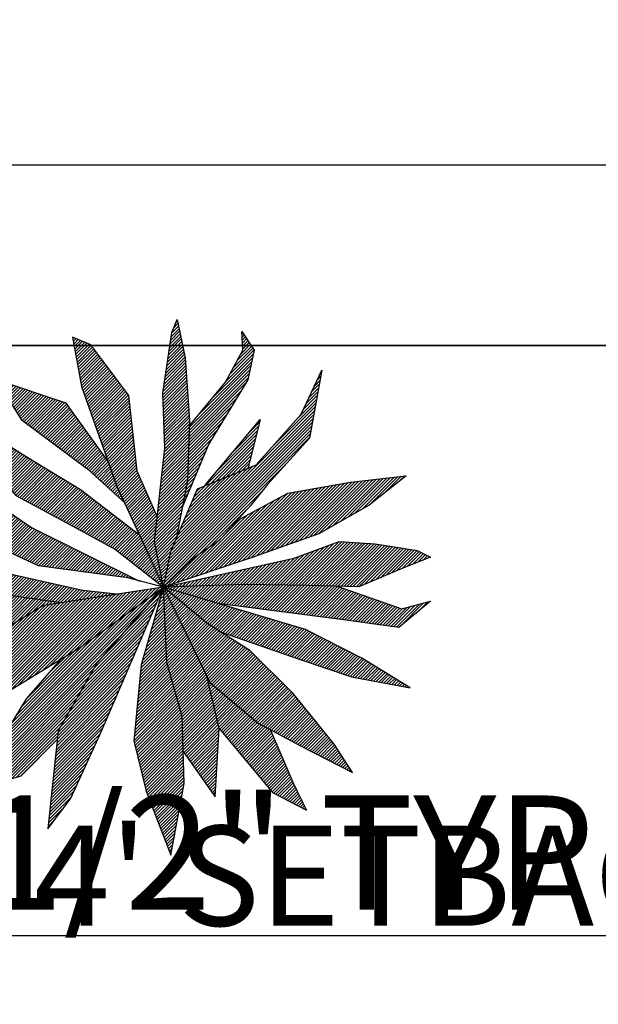
# Model space of a CAD drawing. Units: inches. Extents: x 1986 to 21484, y -1816 to 2016.
# Tile 49 of 85: x 3604 to 3645, y 1855 to 1924. Entities that reach past the tile are written whole.
import ezdxf

# ---------------------------------------------------------------- set-up
doc = ezdxf.new("R2010")
doc.units = ezdxf.units.IN
for name, color, linetype, lineweight in [('A-ANNO-DIMS', 2, 'Continuous', 18), ('A-ANNO-TEXT', 7, 'Continuous', 18), ('C-PROP', 7, 'Continuous', 35), ('L-PLNT', 84, 'Continuous', 13), ('vfolhas', 114, 'Continuous', 5)]:
    doc.layers.add(name, color=color, linetype=linetype, lineweight=lineweight)
for name, color, linetype in [('vfolha', 72, 'Continuous'), ('vfolha2', 110, 'Continuous'), ('vfolhas2', 102, 'Continuous')]:
    doc.layers.add(name, color=color, linetype=linetype)
doc.styles.get("Standard").update_dxf_attribs({"font": 'arial.ttf'})
doc.dimstyles.new('ISO-25', dxfattribs={"dimtxt": 8, "dimasz": 2.5, "dimexe": 1.25, "dimexo": 0.625, "dimtad": 1, "dimdec": 1, "dimlunit": 3, "dimtxsty": 'Standard', "dimcen": 2.5, "dimadec": 0, "dimazin": 0, "dimtfac": 1, "dimtdec": 1, "dimtmove": 0, "dimatfit": 3, "dimfxl": 1, "dimarcsym": 0})
pattern_1 = [(45, (-2446.5133113, 50.986076), (-0.004419417382, 0.004419417382), [])]

# ---------------------------------------------------------------- blocks, each defined once
blk = doc.blocks.new('*D33')
at = {"layer": 'A-ANNO-DIMS', "color": 0, "lineweight": -2, "transparency": 16777216}
for p, q in [((3538.907, 1901.377), (3538.907, 1914.655)), ((3898.907, 1901.377), (3898.907, 1914.655)), ((3541.407, 1913.405), (3896.407, 1913.405))]:
    blk.add_line(p, q, dxfattribs=at)
at = {"layer": 'A-ANNO-DIMS', "color": 0, "transparency": 16777216}
for points in [[(3541.407, 1913.821), (3541.407, 1912.988), (3538.907, 1913.405)], [(3896.407, 1913.821), (3896.407, 1912.988), (3898.907, 1913.405)]]:
    blk.add_solid(points, dxfattribs=at)
at = {"layer": 'Defpoints', "color": 0, "transparency": 16777216}
for p in [(3898.907, 1913.405), (3538.907, 1900.752), (3898.907, 1900.752)]:
    blk.add_point(p, dxfattribs=at)
at = {"layer": 'A-ANNO-DIMS', "color": 0, "transparency": 16777216, "insert": (3718.907, 1918.117), "char_height": 8, "attachment_point": 5}
blk.add_mtext("30'", dxfattribs=at)
blk = doc.blocks.new('arbusto_PB_verde_grande')
at = {"layer": 'vfolha2'}
h = blk.add_hatch(dxfattribs=at)
h.set_pattern_fill('ANSI31', color=256, scale=0.05, style=0)
h.set_pattern_definition(pattern_1)
h.paths.add_polyline_path([(0.0294, 0.3565), (0.0003, 0.0905), (0.0263, -0.0393), (0.047, 0.0623), (0.0619, 0.0973), (0.0937, 0.2657), (0.0996, 0.4347), (0.0879, 0.6131), (0.0645, 0.7227), (0.0499, 0.6851), (0.0236, 0.5129)])
h.paths.add_polyline_path([(0.3011, 0.4379), (0.1423, 0.2487), (0.2669, 0.3002)])
h.paths.add_polyline_path([(0.38, 0.2282), (0.237, 0.1519), (0.1843, 0.0936), (0.1112, 0.0436), (0.0263, -0.0393), (0.2806, 0.0467), (0.3683, 0.078), (0.4676, 0.1124), (0.6107, 0.1938), (0.7159, 0.2782), (0.5581, 0.2595)])
h.paths.add_polyline_path([(0.561, -0.2944), (0.7275, -0.3257), (0.5902, -0.2412), (0.4296, -0.1598), (0.0263, -0.0393), (0.1492, -0.1411), (0.1884, -0.166), (0.415, -0.2444)])
h.paths.add_polyline_path([(-0.2743, -0.4478), (-0.3035, -0.7263), (-0.2392, -0.6417), (-0.1546, -0.4572), (0.0263, -0.0393), (-0.1633, -0.2538)])
h.paths.add_polyline_path([(-0.5196, -0.2474), (-0.6774, -0.3257), (-0.5956, -0.3507), (-0.4057, -0.3288), (-0.2101, -0.21), (0.0263, -0.0393), (-0.1487, -0.0659), (-0.3152, -0.091), (-0.4145, -0.1505)])
h.paths.add_polyline_path([(-0.5255, 0.2501), (-0.7095, 0.247), (-0.5196, 0.1093), (-0.3298, 0.0217), (-0.0757, -0.0128), (-0.0423, -0.0215), (-0.3502, 0.1312)])
h = blk.add_hatch(dxfattribs=at)
h.set_pattern_fill('ANSI31', color=256, scale=0.05, style=0)
h.set_pattern_definition(pattern_1)
h.paths.add_polyline_path([(-0.1896, 0.297), (-0.0855, 0.2019), (-0.1078, 0.2501), (-0.132, 0.3187), (-0.251, 0.4848), (-0.4495, 0.5505), (-0.3795, 0.4379)])
h.paths.add_polyline_path([(0.0791, -0.4071), (0.0821, -0.5063), (0.1726, -0.6355), (0.1843, -0.4415), (0.149, -0.2918), (0.0263, -0.0393), (0.0353, -0.2538)])
at = {"layer": 'vfolhas'}
h = blk.add_hatch(dxfattribs=at)
h.set_pattern_fill('ANSI31', color=256, scale=0.05, style=0)
h.set_pattern_definition(pattern_1)
h.paths.add_polyline_path([(-0.0728, 0.5067), (-0.1808, 0.6506), (-0.2334, 0.6725), (-0.2071, 0.5318), (-0.1078, 0.2501), (0.0263, -0.0393), (0.0003, 0.0905), (0.0082, 0.1624), (-0.0494, 0.2908)])
h.paths.add_polyline_path([(0.099, 0.4193), (0.0937, 0.2657), (0.0791, 0.1881), (0.1551, 0.369), (0.2661, 0.5505), (0.2836, 0.635), (0.2485, 0.6882), (0.2514, 0.635), (0.2018, 0.5443)])
h.paths.add_polyline_path([(0.1229, 0.2407), (0.047, 0.0623), (0.0263, -0.0393), (0.1112, 0.0436), (0.1843, 0.0936), (0.2748, 0.1938), (0.3215, 0.2532), (0.4413, 0.3847), (0.4763, 0.5787), (0.4179, 0.4535), (0.2894, 0.3095)])
h.paths.add_polyline_path([(0.5815, -0.0378), (0.7071, 0.0154), (0.7859, 0.0467), (0.748, 0.0655), (0.6282, 0.0842), (0.526, 0.0905), (0.3974, 0.0436), (0.0263, -0.0393), (0.2573, -0.0315), (0.4383, -0.0347)])
h.paths.add_polyline_path([(0.5202, -0.0365), (0.4383, -0.0347), (0.2573, -0.0315), (0.0263, -0.0393), (0.1796, -0.0852), (0.5377, -0.1317), (0.6954, -0.1536), (0.7859, -0.0785), (0.7041, -0.1004)])
h.paths.add_polyline_path([(0.2719, -0.2193), (0.1492, -0.1411), (0.0263, -0.0393), (0.1579, -0.3101), (0.2952, -0.4258), (0.4179, -0.4916), (0.564, -0.5667), (0.5114, -0.4853), (0.3946, -0.3414)])
h.paths.add_polyline_path([(-0.0582, -0.4759), (-0.0231, -0.6198), (0.047, -0.8013), (0.0849, -0.5979), (0.0791, -0.4071), (0.0353, -0.2538), (0.0263, -0.0393), (-0.0377, -0.26)])
h.paths.add_polyline_path([(-0.2422, 0.1405), (-0.1107, 0.0686), (0.0263, -0.0393), (-0.0423, 0.1087), (-0.2101, 0.2376), (-0.3649, 0.3314), (-0.4787, 0.4034), (-0.543, 0.4629), (-0.4904, 0.3314), (-0.3941, 0.2219)])
h = blk.add_hatch(dxfattribs=at)
h.set_pattern_fill('ANSI31', color=256, scale=0.05, style=0)
h.set_pattern_definition(pattern_1)
h.paths.add_polyline_path([(-0.5722, 0.0623), (-0.7153, 0.103), (-0.6774, 0.0811), (-0.6277, 0.0154), (-0.5635, -0.041), (-0.2646, -0.0834), (-0.1487, -0.0659), (-0.1015, -0.0588), (-0.2042, -0.0472), (-0.4028, -0.0034)])
h.paths.add_polyline_path([(-0.5635, -0.041), (-0.5828, -0.024), (-0.7299, -0.0973), (-0.4334, -0.1679), (-0.4145, -0.1505), (-0.3152, -0.091), (-0.2646, -0.0834)])
h.paths.add_polyline_path([(-0.2769, -0.4727), (-0.2743, -0.4478), (-0.1633, -0.2538), (0.0263, -0.0393), (-0.2101, -0.21), (-0.2672, -0.2447), (-0.3649, -0.357), (-0.4291, -0.4634), (-0.4759, -0.6043), (-0.3795, -0.576)])
h = blk.add_hatch(dxfattribs=at)
h.set_pattern_fill('ANSI31', color=256, scale=0.05, style=0)
h.set_pattern_definition(pattern_1)
h.paths.add_polyline_path([(0.3361, -0.623), (0.4325, -0.6731), (0.3946, -0.5948), (0.3303, -0.4446), (0.2952, -0.4258), (0.1579, -0.3101), (0.149, -0.2918), (0.1843, -0.4415)])
at = {"layer": 'vfolha'}
for p, q in [((0.0263, -0.0393), (-0.1487, -0.0659)), ((0.0263, -0.0393), (-0.0377, -0.26)), ((0.0353, -0.2538), (0.0263, -0.0393)), ((0.5202, -0.0365), (0.7041, -0.1004)), ((0.7859, -0.0785), (0.6954, -0.1536)), ((0.7041, -0.1004), (0.7859, -0.0785)), ((0.5377, -0.1317), (0.1796, -0.0852)), ((0.6954, -0.1536), (0.5377, -0.1317)), ((0.3946, -0.3414), (0.2719, -0.2193)), ((-0.2672, -0.2447), (-0.3649, -0.357)), ((-0.0377, -0.26), (-0.0582, -0.4759)), ((0.0791, -0.4071), (0.0353, -0.2538)), ((0.1579, -0.3101), (0.2952, -0.4258)), ((0.5114, -0.4853), (0.3946, -0.3414)), ((0.0849, -0.5979), (0.0791, -0.4071)), ((0.2952, -0.4258), (0.4179, -0.4916)), ((0.4179, -0.4916), (0.564, -0.5667)), ((0.564, -0.5667), (0.5114, -0.4853)), ((0.047, -0.8013), (0.0849, -0.5979)), ((-0.0231, -0.6198), (0.047, -0.8013))]:
    blk.add_line(p, q, dxfattribs=at)
at = {"layer": 'vfolha2'}
for p, q in [((0.0499, 0.6851), (0.0645, 0.7227)), ((0.0645, 0.7227), (0.0879, 0.6131)), ((0.0236, 0.5129), (0.0499, 0.6851)), ((0.0879, 0.6131), (0.0996, 0.4347)), ((-0.4495, 0.5505), (-0.3795, 0.4379)), ((-0.251, 0.4848), (-0.4495, 0.5505)), ((0.0294, 0.3565), (0.0236, 0.5129)), ((-0.132, 0.3187), (-0.251, 0.4848)), ((-0.3795, 0.4379), (-0.1896, 0.297)), ((0.0996, 0.4347), (0.0937, 0.2657)), ((0.1434, 0.2501), (0.3011, 0.4379)), ((0.3011, 0.4379), (0.2661, 0.297)), ((0.0003, 0.0905), (0.0294, 0.3565)), ((-0.1896, 0.297), (-0.0822, 0.1989)), ((0.38, 0.2282), (0.5581, 0.2595)), ((0.5581, 0.2595), (0.7159, 0.2782)), ((0.7159, 0.2782), (0.6107, 0.1938)), ((-0.7095, 0.247), (-0.5255, 0.2501)), ((-0.5196, 0.1093), (-0.7095, 0.247)), ((-0.5255, 0.2501), (-0.3502, 0.1312)), ((0.237, 0.1519), (0.38, 0.2282)), ((0.6107, 0.1938), (0.4676, 0.1124)), ((-0.3502, 0.1312), (-0.0423, -0.0215)), ((-0.3298, 0.0217), (-0.5196, 0.1093)), ((0.0263, -0.0393), (0.0003, 0.0905)), ((0.3683, 0.078), (0.2806, 0.0467)), ((0.2806, 0.0467), (0.0263, -0.0393)), ((-0.0757, -0.0128), (-0.3298, 0.0217)), ((-0.2101, -0.21), (0.0263, -0.0393)), ((0.0263, -0.0393), (-0.1633, -0.2538)), ((-0.1546, -0.4572), (0.0263, -0.0393)), ((0.4296, -0.1598), (0.0263, -0.0393)), ((0.0263, -0.0393), (0.1579, -0.3101)), ((-0.1487, -0.0659), (-0.3152, -0.091)), ((-0.3152, -0.091), (-0.4145, -0.1505)), ((-0.4145, -0.1505), (-0.5196, -0.2474)), ((0.1884, -0.166), (0.415, -0.2444)), ((0.5902, -0.2412), (0.4296, -0.1598)), ((-0.4057, -0.3288), (-0.2101, -0.21)), ((-0.5196, -0.2474), (-0.6774, -0.3257)), ((0.415, -0.2444), (0.561, -0.2944)), ((0.7275, -0.3257), (0.5902, -0.2412)), ((-0.1633, -0.2538), (-0.2743, -0.4478)), ((0.1843, -0.4415), (0.149, -0.2918)), ((0.561, -0.2944), (0.7275, -0.3257)), ((-0.6774, -0.3257), (-0.5956, -0.3507)), ((-0.5956, -0.3507), (-0.4057, -0.3288)), ((-0.2743, -0.4478), (-0.3035, -0.7263)), ((0.1726, -0.6355), (0.1843, -0.4415)), ((0.0821, -0.5063), (0.1726, -0.6355)), ((-0.3035, -0.7263), (-0.2392, -0.6417))]:
    blk.add_line(p, q, dxfattribs=at)
at = {"layer": 'vfolhas2'}
for p, q in [((-0.2334, 0.6725), (-0.2071, 0.5318)), ((-0.1808, 0.6506), (-0.2334, 0.6725)), ((0.2514, 0.635), (0.2485, 0.6882)), ((0.2485, 0.6882), (0.2836, 0.635)), ((-0.0728, 0.5067), (-0.1808, 0.6506)), ((0.2018, 0.5443), (0.2514, 0.635)), ((0.2836, 0.635), (0.2661, 0.5505)), ((0.4179, 0.4535), (0.4763, 0.5787)), ((0.4763, 0.5787), (0.4413, 0.3847)), ((0.099, 0.4193), (0.2018, 0.5443)), ((0.2661, 0.5505), (0.1551, 0.369)), ((-0.2071, 0.5318), (-0.1078, 0.2501)), ((-0.0494, 0.2908), (-0.0728, 0.5067)), ((-0.543, 0.4629), (-0.4904, 0.3314)), ((-0.4787, 0.4034), (-0.543, 0.4629)), ((0.2894, 0.3095), (0.4179, 0.4535)), ((-0.3649, 0.3314), (-0.4787, 0.4034)), ((0.1551, 0.369), (0.078, 0.1855)), ((0.4413, 0.3847), (0.3215, 0.2532)), ((-0.4904, 0.3314), (-0.3941, 0.2219)), ((-0.2101, 0.2376), (-0.3649, 0.3314)), ((0.1229, 0.2407), (0.2894, 0.3095)), ((0.0082, 0.1624), (-0.0494, 0.2908)), ((0.0937, 0.2657), (0.0619, 0.0973)), ((0.3215, 0.2532), (0.2748, 0.1938)), ((-0.0423, 0.1087), (-0.2101, 0.2376)), ((-0.1078, 0.2501), (0.0263, -0.0393)), ((0.047, 0.0623), (0.1229, 0.2407)), ((-0.3941, 0.2219), (-0.2422, 0.1405)), ((0.2748, 0.1938), (0.1843, 0.0936)), ((-0.2422, 0.1405), (-0.1107, 0.0686)), ((0.4676, 0.1124), (0.3683, 0.078)), ((-0.6774, 0.0811), (-0.7153, 0.103)), ((-0.7153, 0.103), (-0.5722, 0.0623)), ((0.1843, 0.0936), (0.1112, 0.0436)), ((0.3974, 0.0436), (0.526, 0.0905)), ((0.526, 0.0905), (0.6282, 0.0842)), ((0.6282, 0.0842), (0.748, 0.0655)), ((-0.6277, 0.0154), (-0.6774, 0.0811)), ((-0.5722, 0.0623), (-0.4028, -0.0034)), ((-0.1107, 0.0686), (0.0263, -0.0393)), ((0.0263, -0.0393), (0.047, 0.0623)), ((0.748, 0.0655), (0.7859, 0.0467)), ((0.0263, -0.0393), (0.3974, 0.0436)), ((0.1112, 0.0436), (0.0263, -0.0393)), ((0.7859, 0.0467), (0.7071, 0.0154)), ((-0.5635, -0.041), (-0.6277, 0.0154)), ((0.7071, 0.0154), (0.5815, -0.0378)), ((-0.5828, -0.024), (-0.7299, -0.0973)), ((-0.4028, -0.0034), (-0.2042, -0.0472)), ((0.0263, -0.0393), (-0.0757, -0.0128)), ((-0.2646, -0.0834), (-0.5635, -0.041)), ((-0.2042, -0.0472), (-0.0983, -0.0591)), ((0.2573, -0.0315), (0.0263, -0.0393)), ((0.1492, -0.1411), (0.0263, -0.0393)), ((0.4383, -0.0347), (0.2573, -0.0315)), ((0.5815, -0.0378), (0.4383, -0.0347)), ((-0.7299, -0.0973), (-0.4334, -0.1679)), ((0.2719, -0.2193), (0.1492, -0.1411)), ((-0.3649, -0.357), (-0.4291, -0.4634)), ((0.1843, -0.4415), (0.3361, -0.623)), ((0.3946, -0.5948), (0.329, -0.4417)), ((-0.4291, -0.4634), (-0.4759, -0.6043)), ((-0.3795, -0.576), (-0.2769, -0.4727)), ((-0.2392, -0.6417), (-0.1546, -0.4572)), ((-0.0582, -0.4759), (-0.0231, -0.6198)), ((-0.4759, -0.6043), (-0.3795, -0.576)), ((0.4325, -0.6731), (0.3946, -0.5948)), ((0.3361, -0.623), (0.4325, -0.6731))]:
    blk.add_line(p, q, dxfattribs=at)
blk = doc.blocks.new('*D96')
at = {"layer": 'A-ANNO-DIMS', "color": 0, "lineweight": -2, "transparency": 16777216}
for p, q in [((3539.82, 1864.464), (3539.82, 1858.215)), ((3577.115, 1864.464), (3577.115, 1858.215)), ((3542.32, 1859.465), (3574.615, 1859.465)), ((3577.115, 1859.465), (3648.265, 1859.465))]:
    blk.add_line(p, q, dxfattribs=at)
at = {"layer": 'A-ANNO-DIMS', "color": 0, "transparency": 16777216}
for points in [[(3542.32, 1859.882), (3542.32, 1859.048), (3539.82, 1859.465)], [(3574.615, 1859.882), (3574.615, 1859.048), (3577.115, 1859.465)]]:
    blk.add_solid(points, dxfattribs=at)
at = {"layer": 'Defpoints', "color": 0, "transparency": 16777216}
for p in [(3539.82, 1865.089), (3577.115, 1865.089), (3577.115, 1859.465)]:
    blk.add_point(p, dxfattribs=at)
at = {"layer": 'A-ANNO-DIMS', "color": 0, "transparency": 16777216, "insert": (3613.94, 1864.229), "char_height": 8, "attachment_point": 5}
blk.add_mtext('3\'-1 1/2" TYP.', dxfattribs=at)

msp = doc.modelspace()

# ---------------------------------------------------------------- linework, layer by layer
at = {"layer": 'C-PROP'}
msp.add_lwpolyline([(3538.907, 1900.752), (3898.907, 1900.752), (3898.907, 1066.752), (3538.907, 1066.752)], close=True, dxfattribs=at)

# ---------------------------------------------------------------- block references
at = {"layer": 'L-PLNT', "xscale": 24.60366729364114, "yscale": 24.60366729364114, "zscale": 24.60366729364114}
msp.add_blockref('arbusto_PB_verde_grande', (3613.9, 1884.805), dxfattribs=at)

# ---------------------------------------------------------------- texts
at = {"layer": 'A-ANNO-TEXT', "insert": (3605.478, 1867.143), "char_height": 7, "attachment_point": 1}
msp.add_mtext_dynamic_manual_height_columns("{\\fTimes New Roman|b0|i0|c0|p18;4' SETBACK}", width=105.61268, gutter_width=12.5, heights=[0], dxfattribs=at)

# ---------------------------------------------------------------- dimensions: what is measured, and where the dimension line sits
at = {"layer": 'A-ANNO-DIMS'}
dim = msp.add_linear_dim(base=(3898.907, 1913.405), p1=(3538.907, 1900.752), p2=(3898.907, 1900.752), dimstyle='ISO-25', override={"dimclrd": 0, "dimclre": 0, "dimclrt": 0}, dxfattribs=at)
dim.commit()
dim.dimension.update_dxf_attribs({"geometry": '*D33', "text_midpoint": (3718.907, 1918.117)})
dim = msp.add_linear_dim(base=(3577.115, 1859.465), p1=(3539.82, 1865.089), p2=(3577.115, 1865.089), text='<> TYP.', dimstyle='ISO-25', override={"dimdec": 1, "dimrnd": 0, "dimzin": 1, "dimlunit": 4, "dimfrac": 2}, dxfattribs=at)
dim.commit()
dim.dimension.update_dxf_attribs({"geometry": '*D96', "text_midpoint": (3613.94, 1864.229)})

doc.saveas('drawing.dxf')
